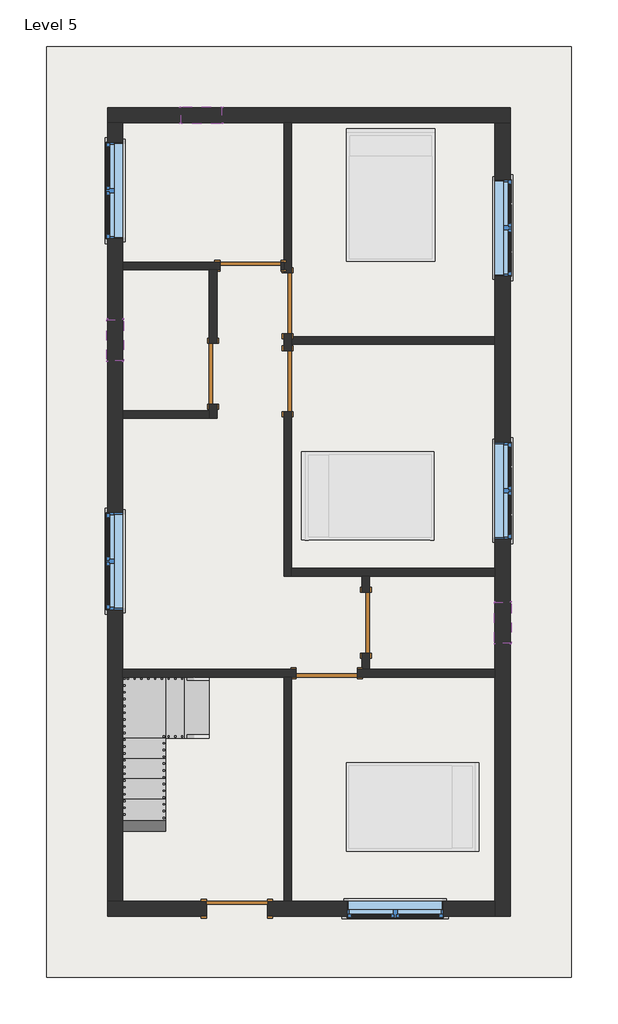
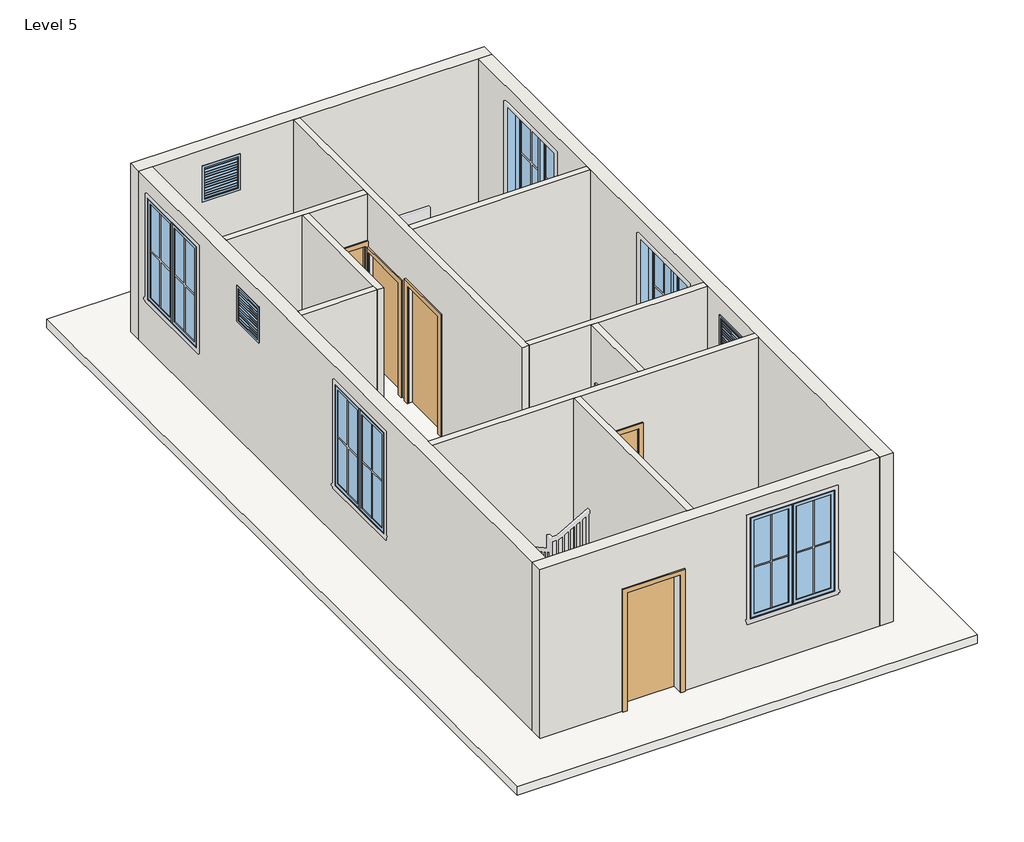
# One storey, part 1 of 2: 13 walls, 8 windows, 7 doors, 1 roof, 1 stair flight.
"""IFC4 building model written with IfcOpenShell, lengths in millimetres."""

from ifc_helpers import new_model, si_unit, frame, origin, place, context, project, spatial, polyline, outline, extrude, faceted_brep, transform, mapped, element, save
from components import door_5e62189b, door_17d80c48, door_e5f9f3c4, door_305aa2a5, door_0ca8825f, window_9ac97e1a, window_f2d8fef0

model = new_model("IFC4")

# Units and contexts
model_context = context("Model", 3, world=origin())
ifc_project = project(units=[si_unit("LENGTHUNIT", "METRE", prefix="MILLI")], contexts=[model_context])

# Site, building, storey
site = spatial("IfcSite", under=ifc_project)
building = spatial("IfcBuilding", under=site)
storey = spatial("IfcBuildingStorey", under=building, Name="Level 5", Elevation=9601.2)

# Doors
placement = place(None, origin())
door_shape = door_5e62189b(model_context)
element("IfcDoor", 1, ObjectType="Single-Flush : 36\" x 80\"", at=placement, inside=storey, context=model_context, shape_type="MappedRepresentation", body=[
    mapped(door_shape, transform((-2690.3389285, 2204.6069249, 9601.2), x_axis=(0.0, -1.0, 0.0), y_axis=(1.0, 0.0, 0.0), z_axis=(0.0, 0.0, 1.0))),
])
element("IfcDoor", 2, ObjectType="Single-Flush : 36\" x 80\"", at=placement, inside=storey, context=model_context, shape_type="MappedRepresentation", body=[
    mapped(door_shape, transform((-404.3389285, -1522.8430751, 9601.2), x_axis=(0.0, 1.0, 0.0), y_axis=(-1.0, 0.0, 0.0), z_axis=(0.0, 0.0, 1.0))),
])
door_2_shape = door_17d80c48(model_context)
element("IfcDoor", 3, ObjectType="Single-Flush : 36\" x 80\"", at=placement, inside=storey, context=model_context, shape_type="MappedRepresentation", body=[
    mapped(door_2_shape, transform((-1572.7389285, 3258.7069249, 9601.2), x_axis=(0.0, -1.0, 0.0), y_axis=(1.0, 0.0, 0.0), z_axis=(0.0, 0.0, 1.0))),
])
door_3_shape = door_e5f9f3c4(model_context)
element("IfcDoor", 4, ObjectType="Single-Flush : 36\" x 84\"", at=placement, inside=storey, context=model_context, shape_type="MappedRepresentation", body=[
    mapped(door_3_shape, transform((-2131.5389285, 3817.5069249, 9601.2), x_axis=(1.0, 0.0, 0.0), y_axis=(0.0, 1.0, 0.0), z_axis=(0.0, 0.0, 1.0))),
])
element("IfcDoor", 5, ObjectType="Single-Flush : 36\" x 84\"", at=placement, inside=storey, context=model_context, shape_type="MappedRepresentation", body=[
    mapped(door_3_shape, transform((-988.5389285, -2278.4930751, 9601.2), x_axis=(-1.0, 0.0, 0.0), y_axis=(0.0, -1.0, 0.0), z_axis=(0.0, 0.0, 1.0))),
])
door_4_shape = door_305aa2a5(model_context)
element("IfcDoor", 6, ObjectType="Single-Flush : 36\" x 84\"", at=placement, inside=storey, context=model_context, shape_type="MappedRepresentation", body=[
    mapped(door_4_shape, transform((-1572.7389285, 2090.3069249, 9601.2), x_axis=(0.0, 1.0, 0.0), y_axis=(-1.0, 0.0, 0.0), z_axis=(0.0, 0.0, 1.0))),
])
door_5_shape = door_0ca8825f(model_context)
element("IfcDoor", 7, ObjectType="Single-Flush : 36\" x 84\"", at=placement, inside=storey, context=model_context, shape_type="MappedRepresentation", body=[
    mapped(door_5_shape, transform((-2334.7389285, -5802.7430751, 9601.2), x_axis=(1.0, 0.0, 0.0), y_axis=(0.0, 1.0, 0.0), z_axis=(0.0, 0.0, 1.0))),
])

# Roof
element("IfcRoof", 8, ObjectType="ROOF 6\"", at=placement, inside=storey, context=model_context, shape_type="SweptSolid", body=[
    extrude(outline(polyline([(-5185.8889285, 7100.4569249), (2675.4110715, 7100.4569249), (2675.4110715, -6831.4430751), (-5185.8889285, -6831.4430751), (-5185.8889285, 7100.4569249)])), frame((0.0, 0.0, 9448.8), z_axis=(0.0, 0.0, 1.0), x_axis=(1.0, 0.0, 0.0)), (0.0, 0.0, 1.0), 152.4),
])

# Stair flight
element("IfcStairFlight", 9, ObjectType="3/4\" Nosing", at=placement, inside=storey, context=model_context, shape_type="Brep", body=[
    faceted_brep([(-2747.4889285, -3250.0430751, 9770.5333333), (-2747.4889285, -2335.6430751, 9770.5333333), (-3128.4889285, -2335.6430751, 9770.5333333), (-3128.4889285, -3250.0430751, 9770.5333333), (-3128.4889285, -3250.0430751, 9707.0333333), (-2754.6326785, -3250.0430751, 9707.0333333), (-2754.6326785, -2335.6430751, 9707.0333333), (-3128.4889285, -2335.6430751, 9707.0333333)], [[[0, 1, 2, 3]], [[0, 3, 4, 5]], [[2, 1, 6, 7]], [[1, 0, 5, 6]], [[4, 7, 6, 5]], [[7, 4, 3, 2]]]),
    faceted_brep([(-3128.4889285, -3250.0430751, 9939.8666667), (-3128.4889285, -2335.6430751, 9939.8666667), (-3401.5389285, -2335.6430751, 9939.8666667), (-3401.5389285, -3250.0430751, 9939.8666667), (-3401.5389285, -3250.0430751, 9876.3666667), (-3135.6326785, -3250.0430751, 9876.3666667), (-3135.6326785, -2335.6430751, 9876.3666667), (-3401.5389285, -2335.6430751, 9876.3666667)], [[[0, 1, 2, 3]], [[0, 3, 4, 5]], [[2, 1, 6, 7]], [[1, 0, 5, 6]], [[4, 7, 6, 5]], [[7, 4, 3, 2]]]),
    faceted_brep([(-3401.5389285, -3269.0930751, 10109.2), (-3401.5389285, -3250.0430751, 10109.2), (-3401.5389285, -2335.6430751, 10109.2), (-4042.8889285, -2335.6430751, 10109.2), (-4042.8889285, -3269.0930751, 10109.2), (-3401.5389285, -3269.0930751, 10045.7), (-3401.5389285, -3250.0430751, 10045.7), (-3408.6826785, -3250.0430751, 10045.7), (-3408.6826785, -2335.6430751, 10045.7), (-4042.8889285, -2335.6430751, 10045.7), (-4042.8889285, -3269.0930751, 10045.7), (-3401.5389285, -3250.0430751, 10278.5333333), (-4042.8889285, -3250.0430751, 10278.5333333), (-4042.8889285, -3285.5502386, 10278.5333333), (-4042.8889285, -3573.8930751, 10278.5333333), (-3401.5389285, -3573.8930751, 10278.5333333), (-3401.5389285, -3285.5502386, 10278.5333333), (-3401.5389285, -3573.8930751, 10205.9200976), (-3401.5389285, -3285.5502386, 10045.7), (-4042.8889285, -3285.5502386, 10045.7), (-4042.8889285, -3573.8930751, 10205.9200976), (-3401.5389285, -3554.8430751, 10447.8666667), (-4042.8889285, -3554.8430751, 10447.8666667), (-4042.8889285, -3878.6930751, 10447.8666667), (-3401.5389285, -3878.6930751, 10447.8666667), (-3401.5389285, -3878.6930751, 10375.2847552), (-4042.8889285, -3878.6930751, 10375.2847552), (-3401.5389285, -3859.6430751, 10617.2), (-4042.8889285, -3859.6430751, 10617.2), (-4042.8889285, -4183.4930751, 10617.2), (-3401.5389285, -4183.4930751, 10617.2), (-3401.5389285, -4183.4930751, 10544.6494128), (-4042.8889285, -4183.4930751, 10544.6494128), (-3401.5389285, -4164.4430751, 10786.5333333), (-4042.8889285, -4164.4430751, 10786.5333333), (-4042.8889285, -4488.2930751, 10786.5333333), (-3401.5389285, -4488.2930751, 10786.5333333), (-3401.5389285, -4488.2930751, 10714.0140703), (-4042.8889285, -4488.2930751, 10714.0140703), (-3401.5389285, -4792.8112092, 10955.8666667), (-3401.5389285, -4469.2430751, 10955.8666667), (-4042.8889285, -4469.2430751, 10955.8666667), (-4042.8889285, -4792.8112092, 10955.8666667), (-3401.5389285, -4773.7612092, 11125.2), (-3401.5389285, -5114.0119996, 11125.2), (-3401.5389285, -5114.0119996, 11061.7), (-4042.8889285, -4792.8112092, 10883.2221068), (-4042.8889285, -4773.7612092, 11125.2), (-4042.8889285, -5114.0119996, 11125.2), (-4042.8889285, -5688.4430751, 11125.2), (-3401.5389285, -5688.4430751, 11125.2), (-4042.8889285, -5114.0119996, 11061.7), (-4042.8889285, -5688.4430751, 11061.7), (-3401.5389285, -5688.4430751, 11061.7)], [[[0, 1, 2, 3, 4]], [[1, 0, 5, 6]], [[7, 1, 6]], [[3, 2, 8, 9]], [[4, 3, 9, 10]], [[11, 12, 13, 14, 15, 16]], [[0, 11, 16, 15, 17, 18, 5]], [[12, 4, 10, 19, 20, 14, 13]], [[21, 22, 23, 24]], [[21, 24, 25, 17, 15]], [[23, 22, 14, 20, 26]], [[27, 28, 29, 30]], [[27, 30, 31, 25, 24]], [[29, 28, 23, 26, 32]], [[33, 34, 35, 36]], [[33, 36, 37, 31, 30]], [[35, 34, 29, 32, 38]], [[39, 40, 41, 42]], [[39, 43, 44, 45, 37, 36, 40]], [[42, 41, 35, 38, 46]], [[43, 47, 48, 49, 50, 44]], [[47, 42, 46, 51, 52, 49, 48]], [[50, 49, 52, 53]], [[2, 1, 7, 8]], [[0, 4, 12, 11]], [[15, 14, 22, 21]], [[24, 23, 28, 27]], [[30, 29, 34, 33]], [[36, 35, 41, 40]], [[39, 42, 47, 43]], [[18, 19, 10, 9, 8, 7, 6, 5]], [[19, 18, 17, 25, 31, 37, 45, 51, 46, 38, 32, 26, 20]], [[45, 53, 52, 51]], [[53, 45, 44, 50]]]),
    faceted_brep([(-3401.5389285, -4773.7612092, 11294.5333333), (-3401.5389285, -5688.4430751, 11294.5333333), (-3128.4889285, -5688.4430751, 11294.5333333), (-3128.4889285, -4773.7612092, 11294.5333333), (-3394.3951785, -4773.7612092, 11231.0333333), (-3128.4889285, -4773.7612092, 11231.0333333), (-3394.3951785, -5688.4430751, 11231.0333333), (-3128.4889285, -5688.4430751, 11231.0333333)], [[[0, 1, 2, 3]], [[4, 0, 3, 5]], [[2, 1, 6, 7]], [[1, 0, 4, 6]], [[5, 7, 6, 4]], [[7, 5, 3, 2]]]),
    faceted_brep([(-3128.4889285, -4773.7612092, 11463.8666667), (-3128.4889285, -5688.4430751, 11463.8666667), (-2793.6303845, -5688.4430751, 11463.8666667), (-2793.6303845, -4773.7612092, 11463.8666667), (-2793.6303845, -4773.7612092, 11400.3666667), (-3121.3451785, -4773.7612092, 11400.3666667), (-3121.3451785, -5688.4430751, 11400.3666667), (-2793.6303845, -5688.4430751, 11400.3666667)], [[[0, 1, 2, 3]], [[0, 3, 4, 5]], [[2, 1, 6, 7]], [[3, 2, 7, 4]], [[1, 0, 5, 6]], [[6, 5, 4, 7]]]),
])

# Walls
element("IfcWall", 10, ObjectType="WALL 4.5\"", at=placement, inside=storey, context=model_context, shape_type="Brep", body=[
    faceted_brep([(-1629.8889285, 2801.5069249, 11633.2), (-1629.8889285, 2801.5069249, 9601.2), (-1629.8889285, 2547.5069249, 9601.2), (-1629.8889285, 2547.5069249, 11734.8), (-1629.8889285, 1633.1069249, 11734.8), (-1629.8889285, 1633.1069249, 9601.2), (-1629.8889285, -824.3430751, 9601.2), (-1629.8889285, -824.3430751, 12649.2), (-1629.8889285, 3760.3569249, 12649.2), (-1629.8889285, 3874.6569249, 12649.2), (-1629.8889285, 5957.4569249, 12649.2), (-1629.8889285, 5957.4569249, 9601.2), (-1629.8889285, 3874.6569249, 9601.2), (-1629.8889285, 3760.3569249, 9601.2), (-1629.8889285, 3715.9069249, 9601.2), (-1629.8889285, 3715.9069249, 11633.2), (-1515.5889285, 2547.5069249, 9601.2), (-1515.5889285, 2642.7569249, 9601.2), (-1515.5889285, 2757.0569249, 9601.2), (-1515.5889285, 2801.5069249, 9601.2), (-1515.5889285, 2801.5069249, 11633.2), (-1515.5889285, 3715.9069249, 11633.2), (-1515.5889285, 3715.9069249, 9601.2), (-1515.5889285, 5957.4569249, 9601.2), (-1515.5889285, 5957.4569249, 12649.2), (-1515.5889285, 2757.0569249, 12649.2), (-1515.5889285, 2642.7569249, 12649.2), (-1515.5889285, -710.0430751, 12649.2), (-1515.5889285, -824.3430751, 12649.2), (-1515.5889285, -824.3430751, 9601.2), (-1515.5889285, -710.0430751, 9601.2), (-1515.5889285, 1633.1069249, 9601.2), (-1515.5889285, 1633.1069249, 11734.8), (-1515.5889285, 2547.5069249, 11734.8)], [[[0, 1, 2, 3, 4, 5, 6, 7, 8, 9, 10, 11, 12, 13, 14, 15]], [[16, 17, 18, 19, 20, 21, 22, 23, 24, 25, 26, 27, 28, 29, 30, 31, 32, 33]], [[31, 30, 29, 6, 5]], [[2, 1, 19, 18, 17, 16]], [[14, 13, 12, 11, 23, 22]], [[11, 10, 24, 23]], [[3, 2, 16, 33]], [[4, 3, 33, 32]], [[5, 4, 32, 31]], [[20, 19, 1, 0]], [[21, 20, 0, 15]], [[22, 21, 15, 14]], [[10, 9, 8, 7, 28, 27, 26, 25, 24]], [[7, 6, 29, 28]]]),
])
element("IfcWall", 11, ObjectType="WALL 4.5\"", at=placement, inside=storey, context=model_context, shape_type="Brep", body=[
    faceted_brep([(1532.4110715, -710.0430751, 9601.2), (-1515.5889285, -710.0430751, 9601.2), (-1515.5889285, -710.0430751, 12649.2), (1532.4110715, -710.0430751, 12649.2), (1532.4110715, -824.3430751, 9601.2), (1532.4110715, -824.3430751, 12649.2), (-347.1889285, -824.3430751, 12649.2), (-461.4889285, -824.3430751, 12649.2), (-1515.5889285, -824.3430751, 12649.2), (-1515.5889285, -824.3430751, 9601.2), (-461.4889285, -824.3430751, 9601.2), (-347.1889285, -824.3430751, 9601.2)], [[[0, 1, 2, 3]], [[4, 5, 6, 7, 8, 9, 10, 11]], [[1, 0, 4, 11, 10, 9]], [[0, 3, 5, 4]], [[3, 2, 8, 7, 6, 5]], [[2, 1, 9, 8]]]),
])
element("IfcWall", 12, ObjectType="WALL 4.5\"", at=placement, inside=storey, context=model_context, shape_type="SweptSolid", body=[
    extrude(outline(polyline([(-1515.5889285, 2757.0569249), (1532.4110715, 2757.0569249), (1532.4110715, 2642.7569249), (-1515.5889285, 2642.7569249), (-1515.5889285, 2757.0569249)])), frame((0.0, 0.0, 9601.2), z_axis=(0.0, 0.0, 1.0), x_axis=(1.0, 0.0, 0.0)), (0.0, 0.0, 1.0), 3048.0),
])
element("IfcWall", 13, ObjectType="WALL 4.5\"", at=placement, inside=storey, context=model_context, shape_type="Brep", body=[
    faceted_brep([(-1674.3389285, 3760.3569249, 11734.8), (-1674.3389285, 3760.3569249, 9601.2), (-1629.8889285, 3760.3569249, 9601.2), (-1629.8889285, 3760.3569249, 12649.2), (-2633.1889285, 3760.3569249, 12649.2), (-2747.4889285, 3760.3569249, 12649.2), (-4042.8889285, 3760.3569249, 12649.2), (-4042.8889285, 3760.3569249, 9601.2), (-2747.4889285, 3760.3569249, 9601.2), (-2633.1889285, 3760.3569249, 9601.2), (-2588.7389285, 3760.3569249, 9601.2), (-2588.7389285, 3760.3569249, 11734.8), (-1629.8889285, 3874.6569249, 9601.2), (-1674.3389285, 3874.6569249, 9601.2), (-1674.3389285, 3874.6569249, 11734.8), (-2588.7389285, 3874.6569249, 11734.8), (-2588.7389285, 3874.6569249, 9601.2), (-4042.8889285, 3874.6569249, 9601.2), (-4042.8889285, 3874.6569249, 12649.2), (-1629.8889285, 3874.6569249, 12649.2)], [[[0, 1, 2, 3, 4, 5, 6, 7, 8, 9, 10, 11]], [[12, 13, 14, 15, 16, 17, 18, 19]], [[2, 1, 13, 12]], [[10, 9, 8, 7, 17, 16]], [[7, 6, 18, 17]], [[3, 2, 12, 19]], [[14, 13, 1, 0]], [[15, 14, 0, 11]], [[16, 15, 11, 10]], [[6, 5, 4, 3, 19, 18]]]),
])
element("IfcWall", 14, ObjectType="WALL 4.5\"", at=placement, inside=storey, context=model_context, shape_type="Brep", body=[
    faceted_brep([(-2747.4889285, 1747.4069249, 11633.2), (-2747.4889285, 1747.4069249, 9601.2), (-2747.4889285, 1652.1569249, 9601.2), (-2747.4889285, 1537.8569249, 9601.2), (-2747.4889285, 1537.8569249, 12649.2), (-2747.4889285, 1652.1569249, 12649.2), (-2747.4889285, 3760.3569249, 12649.2), (-2747.4889285, 3760.3569249, 9601.2), (-2747.4889285, 2661.8069249, 9601.2), (-2747.4889285, 2661.8069249, 11633.2), (-2633.1889285, 1537.8569249, 9601.2), (-2633.1889285, 1747.4069249, 9601.2), (-2633.1889285, 1747.4069249, 11633.2), (-2633.1889285, 2661.8069249, 11633.2), (-2633.1889285, 2661.8069249, 9601.2), (-2633.1889285, 3760.3569249, 9601.2), (-2633.1889285, 3760.3569249, 12649.2), (-2633.1889285, 1537.8569249, 12649.2)], [[[0, 1, 2, 3, 4, 5, 6, 7, 8, 9]], [[10, 11, 12, 13, 14, 15, 16, 17]], [[8, 7, 15, 14]], [[3, 2, 1, 11, 10]], [[7, 6, 16, 15]], [[4, 3, 10, 17]], [[12, 11, 1, 0]], [[13, 12, 0, 9]], [[14, 13, 9, 8]], [[6, 5, 4, 17, 16]]]),
])
element("IfcWall", 15, ObjectType="WALL 4.5\"", at=placement, inside=storey, context=model_context, shape_type="SweptSolid", body=[
    extrude(outline(polyline([(-4042.8889285, 1652.1569249), (-2747.4889285, 1652.1569249), (-2747.4889285, 1537.8569249), (-4042.8889285, 1537.8569249), (-4042.8889285, 1652.1569249)])), frame((0.0, 0.0, 9601.2), z_axis=(0.0, 0.0, 1.0), x_axis=(1.0, 0.0, 0.0)), (0.0, 0.0, 1.0), 3048.0),
])
element("IfcWall", 16, ObjectType="WALL 4.5\"", at=placement, inside=storey, context=model_context, shape_type="Brep", body=[
    faceted_brep([(-4042.8889285, -2335.6430751, 9601.2), (-1629.8889285, -2335.6430751, 9601.2), (-1515.5889285, -2335.6430751, 9601.2), (-1445.7389285, -2335.6430751, 9601.2), (-1445.7389285, -2335.6430751, 11734.8), (-531.3389285, -2335.6430751, 11734.8), (-531.3389285, -2335.6430751, 9601.2), (1532.4110715, -2335.6430751, 9601.2), (1532.4110715, -2335.6430751, 12649.2), (-1515.5889285, -2335.6430751, 12649.2), (-1629.8889285, -2335.6430751, 12649.2), (-4042.8889285, -2335.6430751, 12649.2), (-1445.7389285, -2221.3430751, 11734.8), (-1445.7389285, -2221.3430751, 9601.2), (-4042.8889285, -2221.3430751, 9601.2), (-4042.8889285, -2221.3430751, 12649.2), (-461.4889285, -2221.3430751, 12649.2), (-347.1889285, -2221.3430751, 12649.2), (1532.4110715, -2221.3430751, 12649.2), (1532.4110715, -2221.3430751, 9601.2), (-347.1889285, -2221.3430751, 9601.2), (-461.4889285, -2221.3430751, 9601.2), (-531.3389285, -2221.3430751, 9601.2), (-531.3389285, -2221.3430751, 11734.8)], [[[0, 1, 2, 3, 4, 5, 6, 7, 8, 9, 10, 11]], [[12, 13, 14, 15, 16, 17, 18, 19, 20, 21, 22, 23]], [[14, 13, 3, 2, 1, 0]], [[22, 21, 20, 19, 7, 6]], [[8, 7, 19, 18]], [[0, 11, 15, 14]], [[4, 3, 13, 12]], [[5, 4, 12, 23]], [[6, 5, 23, 22]], [[11, 10, 9, 8, 18, 17, 16, 15]]]),
])
element("IfcWall", 17, ObjectType="WALL 4.5\"", at=placement, inside=storey, context=model_context, shape_type="SweptSolid", body=[
    extrude(outline(polyline([(-824.3430751, 9601.2), (-1065.6430751, 9601.2), (-1065.6430751, 11633.2), (-1980.0430751, 11633.2), (-1980.0430751, 9601.2), (-2221.3430751, 9601.2), (-2221.3430751, 12649.2), (-824.3430751, 12649.2), (-824.3430751, 9601.2)])), frame((-461.4889285, 0.0, 0.0), z_axis=(1.0, 0.0, 0.0), x_axis=(0.0, 1.0, 0.0)), (0.0, 0.0, 1.0), 114.3),
])
element("IfcWall", 18, ObjectType="WALL 4.5\"", at=placement, inside=storey, context=model_context, shape_type="SweptSolid", body=[
    extrude(outline(polyline([(-1629.8889285, -5688.4430751), (-1629.8889285, -2335.6430751), (-1515.5889285, -2335.6430751), (-1515.5889285, -5688.4430751), (-1629.8889285, -5688.4430751)])), frame((0.0, 0.0, 9601.2), z_axis=(0.0, 0.0, 1.0), x_axis=(1.0, 0.0, 0.0)), (0.0, 0.0, 1.0), 3048.0),
])
element("IfcWall", 19, ObjectType="WALL 9\"", at=placement, inside=storey, context=model_context, shape_type="Brep", body=[
    faceted_brep([(-4271.4889285, 5957.4569249, 9601.2), (-4042.8889285, 5957.4569249, 9601.2), (-1629.8889285, 5957.4569249, 9601.2), (-1515.5889285, 5957.4569249, 9601.2), (1532.4110715, 5957.4569249, 9601.2), (1761.0110715, 5957.4569249, 9601.2), (1761.0110715, 5957.4569249, 12649.2), (1532.4110715, 5957.4569249, 12649.2), (-1515.5889285, 5957.4569249, 12649.2), (-1629.8889285, 5957.4569249, 12649.2), (-4042.8889285, 5957.4569249, 12649.2), (-4271.4889285, 5957.4569249, 12649.2), (-2560.1639285, 5957.4569249, 12344.4), (-2560.1639285, 5957.4569249, 11734.8), (-3169.7639285, 5957.4569249, 11734.8), (-3169.7639285, 5957.4569249, 12344.4), (-4271.4889285, 6186.0569249, 9601.2), (-4271.4889285, 6186.0569249, 12649.2), (1761.0110715, 6186.0569249, 12649.2), (1761.0110715, 6186.0569249, 9601.2), (-2560.1639285, 6186.0569249, 12344.4), (-3169.7639285, 6186.0569249, 12344.4), (-3169.7639285, 6186.0569249, 11734.8), (-2560.1639285, 6186.0569249, 11734.8)], [[[0, 1, 2, 3, 4, 5, 6, 7, 8, 9, 10, 11], [12, 13, 14, 15]], [[16, 17, 18, 19], [20, 21, 22, 23]], [[5, 4, 3, 2, 1, 0, 16, 19]], [[6, 5, 19, 18]], [[0, 11, 17, 16]], [[13, 12, 20, 23]], [[14, 13, 23, 22]], [[15, 14, 22, 21]], [[12, 15, 21, 20]], [[11, 10, 9, 8, 7, 6, 18, 17]]]),
])
element("IfcWall", 20, ObjectType="WALL 9\"", at=placement, inside=storey, context=model_context, shape_type="Brep", body=[
    faceted_brep([(1532.4110715, 5957.4569249, 9601.2), (1532.4110715, 2757.0569249, 9601.2), (1532.4110715, 2642.7569249, 9601.2), (1532.4110715, -710.0430751, 9601.2), (1532.4110715, -824.3430751, 9601.2), (1532.4110715, -2221.3430751, 9601.2), (1532.4110715, -2335.6430751, 9601.2), (1532.4110715, -5688.4430751, 9601.2), (1532.4110715, -5917.0430751, 9601.2), (1532.4110715, -5917.0430751, 12649.2), (1532.4110715, -5688.4430751, 12649.2), (1532.4110715, -2335.6430751, 12649.2), (1532.4110715, -2221.3430751, 12649.2), (1532.4110715, -824.3430751, 12649.2), (1532.4110715, -710.0430751, 12649.2), (1532.4110715, 2642.7569249, 12649.2), (1532.4110715, 2757.0569249, 12649.2), (1532.4110715, 5957.4569249, 12649.2), (1532.4110715, 3661.9319249, 12344.4), (1532.4110715, 3661.9319249, 10515.6), (1532.4110715, 5109.7319249, 10515.6), (1532.4110715, 5109.7319249, 12344.4), (1532.4110715, -271.8930751, 12344.4), (1532.4110715, -271.8930751, 10515.6), (1532.4110715, 1175.9069249, 10515.6), (1532.4110715, 1175.9069249, 12344.4), (1532.4110715, -1827.6430751, 12344.4), (1532.4110715, -1827.6430751, 11734.8), (1532.4110715, -1218.0430751, 11734.8), (1532.4110715, -1218.0430751, 12344.4), (1761.0110715, 5957.4569249, 9601.2), (1761.0110715, 5957.4569249, 12649.2), (1761.0110715, -5917.0430751, 12649.2), (1761.0110715, -5917.0430751, 9601.2), (1761.0110715, 3661.9319249, 12344.4), (1761.0110715, 5109.7319249, 12344.4), (1761.0110715, 5109.7319249, 10515.6), (1761.0110715, 3661.9319249, 10515.6), (1761.0110715, -271.8930751, 12344.4), (1761.0110715, 1175.9069249, 12344.4), (1761.0110715, 1175.9069249, 10515.6), (1761.0110715, -271.8930751, 10515.6), (1761.0110715, -1827.6430751, 12344.4), (1761.0110715, -1218.0430751, 12344.4), (1761.0110715, -1218.0430751, 11734.8), (1761.0110715, -1827.6430751, 11734.8)], [[[0, 1, 2, 3, 4, 5, 6, 7, 8, 9, 10, 11, 12, 13, 14, 15, 16, 17], [18, 19, 20, 21], [22, 23, 24, 25], [26, 27, 28, 29]], [[30, 31, 32, 33], [34, 35, 36, 37], [38, 39, 40, 41], [42, 43, 44, 45]], [[8, 7, 6, 5, 4, 3, 2, 1, 0, 30, 33]], [[0, 17, 31, 30]], [[9, 8, 33, 32]], [[19, 18, 34, 37]], [[20, 19, 37, 36]], [[21, 20, 36, 35]], [[18, 21, 35, 34]], [[23, 22, 38, 41]], [[24, 23, 41, 40]], [[25, 24, 40, 39]], [[22, 25, 39, 38]], [[27, 26, 42, 45]], [[28, 27, 45, 44]], [[29, 28, 44, 43]], [[26, 29, 43, 42]], [[17, 16, 15, 14, 13, 12, 11, 10, 9, 32, 31]]]),
])
element("IfcWall", 21, ObjectType="WALL 9\"", at=placement, inside=storey, context=model_context, shape_type="Brep", body=[
    faceted_brep([(1532.4110715, -5688.4430751, 9601.2), (-1515.5889285, -5688.4430751, 9601.2), (-1629.8889285, -5688.4430751, 9601.2), (-1877.5389285, -5688.4430751, 9601.2), (-1877.5389285, -5688.4430751, 11734.8), (-2791.9389285, -5688.4430751, 11734.8), (-2791.9389285, -5688.4430751, 9601.2), (-4042.8889285, -5688.4430751, 9601.2), (-4271.4889285, -5688.4430751, 9601.2), (-4271.4889285, -5688.4430751, 12649.2), (-4042.8889285, -5688.4430751, 12649.2), (-1629.8889285, -5688.4430751, 12649.2), (-1515.5889285, -5688.4430751, 12649.2), (1532.4110715, -5688.4430751, 12649.2), (-686.9139285, -5688.4430751, 12344.4), (-686.9139285, -5688.4430751, 10515.6), (760.8860715, -5688.4430751, 10515.6), (760.8860715, -5688.4430751, 12344.4), (-1877.5389285, -5917.0430751, 11734.8), (-1877.5389285, -5917.0430751, 9601.2), (1532.4110715, -5917.0430751, 9601.2), (1532.4110715, -5917.0430751, 12649.2), (-4271.4889285, -5917.0430751, 12649.2), (-4271.4889285, -5917.0430751, 9601.2), (-2791.9389285, -5917.0430751, 9601.2), (-2791.9389285, -5917.0430751, 11734.8), (-686.9139285, -5917.0430751, 12344.4), (760.8860715, -5917.0430751, 12344.4), (760.8860715, -5917.0430751, 10515.6), (-686.9139285, -5917.0430751, 10515.6)], [[[0, 1, 2, 3, 4, 5, 6, 7, 8, 9, 10, 11, 12, 13], [14, 15, 16, 17]], [[18, 19, 20, 21, 22, 23, 24, 25], [26, 27, 28, 29]], [[24, 23, 8, 7, 6]], [[20, 19, 3, 2, 1, 0]], [[0, 13, 21, 20]], [[9, 8, 23, 22]], [[15, 14, 26, 29]], [[16, 15, 29, 28]], [[17, 16, 28, 27]], [[14, 17, 27, 26]], [[4, 3, 19, 18]], [[5, 4, 18, 25]], [[6, 5, 25, 24]], [[13, 12, 11, 10, 9, 22, 21]]]),
])
element("IfcWall", 22, ObjectType="WALL 9\"", at=placement, inside=storey, context=model_context, shape_type="Brep", body=[
    faceted_brep([(-4042.8889285, -5688.4430751, 9601.2), (-4042.8889285, -2335.6430751, 9601.2), (-4042.8889285, -2221.3430751, 9601.2), (-4042.8889285, 1537.8569249, 9601.2), (-4042.8889285, 1652.1569249, 9601.2), (-4042.8889285, 3760.3569249, 9601.2), (-4042.8889285, 3874.6569249, 9601.2), (-4042.8889285, 5957.4569249, 9601.2), (-4042.8889285, 5957.4569249, 12649.2), (-4042.8889285, 3874.6569249, 12649.2), (-4042.8889285, 3760.3569249, 12649.2), (-4042.8889285, 1652.1569249, 12649.2), (-4042.8889285, 1537.8569249, 12649.2), (-4042.8889285, -2221.3430751, 12649.2), (-4042.8889285, -2335.6430751, 12649.2), (-4042.8889285, -5688.4430751, 12649.2), (-4042.8889285, 5668.5319249, 12344.4), (-4042.8889285, 5668.5319249, 10515.6), (-4042.8889285, 4220.7319249, 10515.6), (-4042.8889285, 4220.7319249, 12344.4), (-4042.8889285, 121.8069249, 12344.4), (-4042.8889285, 121.8069249, 10515.6), (-4042.8889285, -1325.9930751, 10515.6), (-4042.8889285, -1325.9930751, 12344.4), (-4042.8889285, 2401.4569249, 12344.4), (-4042.8889285, 3011.0569249, 12344.4), (-4042.8889285, 3011.0569249, 11734.8), (-4042.8889285, 2401.4569249, 11734.8), (-4271.4889285, -5688.4430751, 9601.2), (-4271.4889285, -5688.4430751, 12649.2), (-4271.4889285, 5957.4569249, 12649.2), (-4271.4889285, 5957.4569249, 9601.2), (-4271.4889285, 5668.5319249, 12344.4), (-4271.4889285, 4220.7319249, 12344.4), (-4271.4889285, 4220.7319249, 10515.6), (-4271.4889285, 5668.5319249, 10515.6), (-4271.4889285, 121.8069249, 12344.4), (-4271.4889285, -1325.9930751, 12344.4), (-4271.4889285, -1325.9930751, 10515.6), (-4271.4889285, 121.8069249, 10515.6), (-4271.4889285, 2401.4569249, 12344.4), (-4271.4889285, 2401.4569249, 11734.8), (-4271.4889285, 3011.0569249, 11734.8), (-4271.4889285, 3011.0569249, 12344.4)], [[[0, 1, 2, 3, 4, 5, 6, 7, 8, 9, 10, 11, 12, 13, 14, 15], [16, 17, 18, 19], [20, 21, 22, 23], [24, 25, 26, 27]], [[28, 29, 30, 31], [32, 33, 34, 35], [36, 37, 38, 39], [40, 41, 42, 43]], [[7, 6, 5, 4, 3, 2, 1, 0, 28, 31]], [[0, 15, 29, 28]], [[8, 7, 31, 30]], [[17, 16, 32, 35]], [[18, 17, 35, 34]], [[19, 18, 34, 33]], [[16, 19, 33, 32]], [[21, 20, 36, 39]], [[22, 21, 39, 38]], [[23, 22, 38, 37]], [[20, 23, 37, 36]], [[41, 40, 24, 27]], [[42, 41, 27, 26]], [[43, 42, 26, 25]], [[40, 43, 25, 24]], [[15, 14, 13, 12, 11, 10, 9, 8, 30, 29]]]),
])

# Windows
window_shape = window_9ac97e1a(model_context)
element("IfcWindow", 23, ObjectType="Window-Casement-Double : 57\" x 72\"", at=placement, inside=storey, context=model_context, shape_type="MappedRepresentation", body=[
    mapped(window_shape, transform((-4157.1889285, 4944.6319249, 9601.2), x_axis=(0.0, 1.0, 0.0), y_axis=(-1.0, 0.0, 0.0), z_axis=(0.0, 0.0, 1.0))),
])
element("IfcWindow", 24, ObjectType="Window-Casement-Double : 57\" x 72\"", at=placement, inside=storey, context=model_context, shape_type="MappedRepresentation", body=[
    mapped(window_shape, transform((1646.7110715, 4385.8319249, 9601.2), x_axis=(0.0, -1.0, 0.0), y_axis=(1.0, 0.0, 0.0), z_axis=(0.0, 0.0, 1.0))),
])
element("IfcWindow", 25, ObjectType="Window-Casement-Double : 57\" x 72\"", at=placement, inside=storey, context=model_context, shape_type="MappedRepresentation", body=[
    mapped(window_shape, transform((-4157.1889285, -602.0930751, 9601.2), x_axis=(0.0, 1.0, 0.0), y_axis=(-1.0, 0.0, 0.0), z_axis=(0.0, 0.0, 1.0))),
])
element("IfcWindow", 26, ObjectType="Window-Casement-Double : 57\" x 72\"", at=placement, inside=storey, context=model_context, shape_type="MappedRepresentation", body=[
    mapped(window_shape, transform((1646.7110715, 452.0069249, 9601.2), x_axis=(0.0, -1.0, 0.0), y_axis=(1.0, 0.0, 0.0), z_axis=(0.0, 0.0, 1.0))),
])
element("IfcWindow", 27, ObjectType="Window-Casement-Double : 57\" x 72\"", at=placement, inside=storey, context=model_context, shape_type="MappedRepresentation", body=[
    mapped(window_shape, transform((36.9860715, -5802.7430751, 9601.2), x_axis=(-1.0, 0.0, 0.0), y_axis=(0.0, -1.0, 0.0), z_axis=(0.0, 0.0, 1.0))),
])
window_2_shape = window_f2d8fef0(model_context)
element("IfcWindow", 28, ObjectType="Window-Louvers : 24\" x 24\"", at=placement, inside=storey, context=model_context, shape_type="MappedRepresentation", body=[
    mapped(window_2_shape, transform((-2864.9639285, 6065.4069249, 10820.4), x_axis=(-1.0, 0.0, 0.0), y_axis=(0.0, -1.0, 0.0), z_axis=(0.0, 0.0, 1.0))),
])
element("IfcWindow", 29, ObjectType="Window-Louvers : 24\" x 24\"", at=placement, inside=storey, context=model_context, shape_type="MappedRepresentation", body=[
    mapped(window_2_shape, transform((-4163.5389285, 2706.2569249, 10820.4), x_axis=(0.0, 1.0, 0.0), y_axis=(-1.0, 0.0, 0.0), z_axis=(0.0, 0.0, 1.0))),
])
element("IfcWindow", 30, ObjectType="Window-Louvers : 24\" x 24\"", at=placement, inside=storey, context=model_context, shape_type="MappedRepresentation", body=[
    mapped(window_2_shape, transform((1640.3610715, -1522.8430751, 10820.4), x_axis=(0.0, 1.0, 0.0), y_axis=(-1.0, 0.0, 0.0), z_axis=(0.0, 0.0, 1.0))),
])

save(model, "model.ifc")

# Revit data of these elements
# Type "Single-Flush : 36\" x 80\""
#   Type Mark = "6"
#   Construction Type Id = "MDOOR"
#   Assembly Code = "C1020"
#   Analytic Construction = "Metal"
#   Thickness = 0' - 2"
#   Heat Transfer Coefficient (U) = 0.651978 BTU/(h·ft²·°F)
#   Height = 6' - 8"
#   Trim Projection Ext = 0' - 1"
#   Trim Projection Int = 0' - 1"
#   Trim Width = 0' - 3"
#   Width = 3' - 0"
#   Define Thermal Properties by = 1
#   Define Thermal Properties by = 1
#   Door Material = Door - Panel
#   Frame Material = Door - Frame
#   Visual Light Transmittance = 0
#   Solar Heat Gain Coefficient = 0
#   Function = (empty or 0)
#   Wall Closure = (empty or 0)
# Type "Single-Flush : 36\" x 84\""
#   Type Mark = "1"
#   Construction Type Id = "MDOOR"
#   Assembly Code = "C1020"
#   Analytic Construction = "Metal"
#   Thickness = 0' - 2"
#   Heat Transfer Coefficient (U) = 0.651978 BTU/(h·ft²·°F)
#   Height = 7' - 0"
#   Trim Projection Ext = 0' - 1"
#   Trim Projection Int = 0' - 1"
#   Trim Width = 0' - 3"
#   Width = 3' - 0"
#   Define Thermal Properties by = 1
#   Define Thermal Properties by = 1
#   Door Material = Door - Panel
#   Frame Material = Door - Frame
#   Visual Light Transmittance = 0
#   Solar Heat Gain Coefficient = 0
#   Function = (empty or 0)
#   Wall Closure = (empty or 0)
# Type "ROOF 6\""
#   Assembly Code = "B1020"
#   Layers, outside or top first: 0' - 6" no material (function 1)
# Type "WALL 4.5\""
#   Assembly Code = "B2010"
#   Layers, outside or top first: 0' - 4 1/2" no material (function 1)
# Type "WALL 9\""
#   Assembly Code = "B2010"
#   Layers, outside or top first: 0' - 9" no material (function 1)
# Type "Window-Casement-Double : 57\" x 72\""
#   Type Mark = "17"
#   Fire Rating = "0.5h"
#   Assembly Code = "B2020100"
#   Analytic Construction = "Double glazing - domestic"
#   Frame Extension [instance default] = 0' - 0 1/4"
#   Window Inset [instance default] = 0' - 0"
#   Wall Thickness [instance default] = 0' - 6"
#   Interior Wall Closure [instance default] = 0' - 2 1/4"
#   Half Width = 2' - 4 1/2"
#   Visual Light Transmittance = 0.81
#   Thermal Resistance (R) = 1.8146 (h·ft²·°F)/BTU
#   Solar Heat Gain Coefficient = 0.76
#   Rough Width = 4' - 9 1/2"
#   Rough Height = 6' - 0 1/2"
#   Height = 6' - 0"
#   Heat Transfer Coefficient (U) = 0.5511 BTU/(h·ft²·°F)
#   Exterior Wall Closure [instance default] = 0' - 1 1/4"
#   Extension Jamb [instance default] = 0' - 2 1/4"
#   Default Sill Height = 3' - 0"
#   Width = 4' - 9"
#   Define Thermal Properties by = 0
#   Muntin Visibility = yes
#   Interior Trim Visibility [instance default] = yes
#   Exterior Trim Visibility [instance default] = yes
#   Extension Jamb Visibility [instance default] = yes
#   Interior Trim Material = Wood - Stained
#   Muntin Pattern = Muntin Pattern_2x2 : Muntin Pattern_2x2
#   Interior Trim = Trim-Window-Interior-Flat : Picture Frame
#   Interior Frame Material = Wood - Stained
#   Glass Panel Material = Glass
#   Exterior Trim Material = Clad - White
#   Exterior Trim = Trim-Window-Exterior-Flat : with Sill
#   Exterior Frame Material = Clad - White
#   Wall Closure = (empty or 0)
# Type "Window-Louvers : 24\" x 24\""
#   Type Mark = "18"
#   Construction Type Id = "GSP4R"
#   Assembly Code = "B20"
#   Analytic Construction = "1/8 in Pilkington single glazing"
#   Visual Light Transmittance = 0.9
#   Thermal Resistance (R) = 1.53941 (h·ft²·°F)/BTU
#   Solar Heat Gain Coefficient = 0.78
#   Max Height = 1' - 11.74264"
#   Height = 2' - 0"
#   Heat Transfer Coefficient (U) = 0.6496 BTU/(h·ft²·°F)
#   Blade Width [instance default] = 1' - 10 1/2"
#   Blade Vertical Thickness = 0' - 0.35355"
#   Blade Thickness = 0' - 0 1/4"
#   Blade Spacing = 0' - 1 1/2"
#   Blade Height = 0' - 1.85355"
#   Blade Depth = 0' - 3"
#   Blade Angle = 45.00°
#   Default Sill Height = 3' - 0"
#   Trim Projection_Exterior = 0' - 0 1/2"
#   Trim Projection_Interior = 0' - 0 1/2"
#   Trim Width_Exterior = 0' - 1 1/2"
#   Trim Width_Interior = 0' - 1 1/2"
#   Width = 2' - 0"
#   Max Blade Count = 12
#   Define Thermal Properties by = 1
#   Blade Count = 12
#   Frame Material = Birch
#   Louver Material = Birch
#   Trim Exterior Material = Birch
#   Trim Interior Material = Birch
#   Wall Closure = (empty or 0)
# Elements 1, 2, 3 (IfcDoor, "Single-Flush : 36\" x 80\"")
#   Phase Created = New Construction
#   Materials on its faces: "Door - Frame", "Door - Panel"
# Elements 4, 5, 6, 7 (IfcDoor, "Single-Flush : 36\" x 84\"")
#   Phase Created = New Construction
#   Materials on its faces: "Door - Frame", "Door - Panel"
# Element 8 (IfcRoof, "ROOF 6\"")
#   built-in parameter 1001705 = 31.5 (stored number, unit not read)
#   built-in parameter 1001701 = -0.5 (stored number, unit not read)
#   built-in parameter 1001710 = 33615
#   Phase Created = New Construction
#   Materials on its faces: "Default Roof", "Door - Panel"
# Element 9 (IfcStairFlight, "3/4\" Nosing")
#   Phase Created = New Construction
#   Materials on its faces: "Concrete, Cast-in-Place gray"
# Elements 10, 11, 12, 13, 14, 15, 16, 17, 18 (IfcWall, "WALL 4.5\"")
#   Top Offset = 0' - 0"
#   Base Offset = 0' - 0"
#   Unconnected Height = 10' - 0"
#   wall height = 10' - 0"
#   Phase Created = New Construction
#   Base Constraint = Level 5
#   Materials on its faces: "Default Wall"
# Elements 19, 20, 21, 22 (IfcWall, "WALL 9\"")
#   Top Offset = 0' - 0"
#   Base Offset = 0' - 0"
#   Unconnected Height = 10' - 0"
#   wall height = 10' - 0"
#   Phase Created = New Construction
#   Base Constraint = Level 5
#   Materials on its faces: "Default Wall", "Copper"
# Element 23 (IfcWindow, "Window-Casement-Double : 57\" x 72\"")
#   Mark = "25"
#   Window Inset = 0' - 0"
#   Interior Wall Closure = 0' - 2 1/4"
#   Frame Extension = 0' - 0 1/4"
#   Exterior Wall Closure = 0' - 1 1/4"
#   Interior Trim Visibility = yes
#   Exterior Trim Visibility = yes
#   Phase Created = New Construction
#   Materials on its faces: "Wood - Stained", "Glass", "Clad - White"
# Element 24 (IfcWindow, "Window-Casement-Double : 57\" x 72\"")
#   Mark = "26"
#   Window Inset = 0' - 0"
#   Interior Wall Closure = 0' - 2 1/4"
#   Frame Extension = 0' - 0 1/4"
#   Exterior Wall Closure = 0' - 1 1/4"
#   Interior Trim Visibility = yes
#   Exterior Trim Visibility = yes
#   Phase Created = New Construction
#   Materials on its faces: "Wood - Stained", "Glass", "Clad - White"
# Element 25 (IfcWindow, "Window-Casement-Double : 57\" x 72\"")
#   Mark = "27"
#   Window Inset = 0' - 0"
#   Interior Wall Closure = 0' - 2 1/4"
#   Frame Extension = 0' - 0 1/4"
#   Exterior Wall Closure = 0' - 1 1/4"
#   Interior Trim Visibility = yes
#   Exterior Trim Visibility = yes
#   Phase Created = New Construction
#   Materials on its faces: "Wood - Stained", "Glass", "Clad - White"
# Element 26 (IfcWindow, "Window-Casement-Double : 57\" x 72\"")
#   Mark = "28"
#   Window Inset = 0' - 0"
#   Interior Wall Closure = 0' - 2 1/4"
#   Frame Extension = 0' - 0 1/4"
#   Exterior Wall Closure = 0' - 1 1/4"
#   Interior Trim Visibility = yes
#   Exterior Trim Visibility = yes
#   Phase Created = New Construction
#   Materials on its faces: "Wood - Stained", "Glass", "Clad - White"
# Element 27 (IfcWindow, "Window-Casement-Double : 57\" x 72\"")
#   Mark = "29"
#   Window Inset = 0' - 0"
#   Interior Wall Closure = 0' - 2 1/4"
#   Frame Extension = 0' - 0 1/4"
#   Exterior Wall Closure = 0' - 1 1/4"
#   Interior Trim Visibility = yes
#   Exterior Trim Visibility = yes
#   Phase Created = New Construction
#   Materials on its faces: "Wood - Stained", "Glass", "Clad - White"
# Element 28 (IfcWindow, "Window-Louvers : 24\" x 24\"")
#   Mark = "30"
#   Blade Width = 1' - 10 1/2"
#   Phase Created = New Construction
#   Materials on its faces: "Birch"
# Element 29 (IfcWindow, "Window-Louvers : 24\" x 24\"")
#   Mark = "31"
#   Blade Width = 1' - 10 1/2"
#   Phase Created = New Construction
#   Materials on its faces: "Birch"
# Element 30 (IfcWindow, "Window-Louvers : 24\" x 24\"")
#   Mark = "32"
#   Blade Width = 1' - 10 1/2"
#   Phase Created = New Construction
#   Materials on its faces: "Birch"
# Materials
#   "Door - Panel": class "Wood", colour RGB 210 159 95, transparency 0, Cost = 0
#   "Door - Frame": colour RGB 118 70 51, transparency 0, Cost = 0
#   "Wood - Stained": class "Wood", colour RGB 224 178 126, transparency 0, Cost = 0
#   "Glass": class "Glass", colour RGB 0 128 192, transparency 0.75, Description = "Soda Lime Glass", Cost = 0
#   "Clad - White": class "Wood", colour RGB 242 242 238, transparency 0, Cost = 0
#   "Birch": class "Wood", colour RGB 224 178 126, transparency 0, Description = "Betula Alleghaniensis", Cost = 0
#   "Default Roof": colour RGB 88 101 114, transparency 0, Cost = 0
#   "Concrete, Cast-in-Place gray": class "Concrete", colour RGB 192 192 192, transparency 0, Description = "Cast-in-place concrete", Cost = 0
#   "Default Wall": colour RGB 128 128 128, transparency 0, Cost = 0
#   "Copper": class "Metal", colour RGB 0 0 0, transparency 0, Description = "Copper, matte finish", Cost = 0
